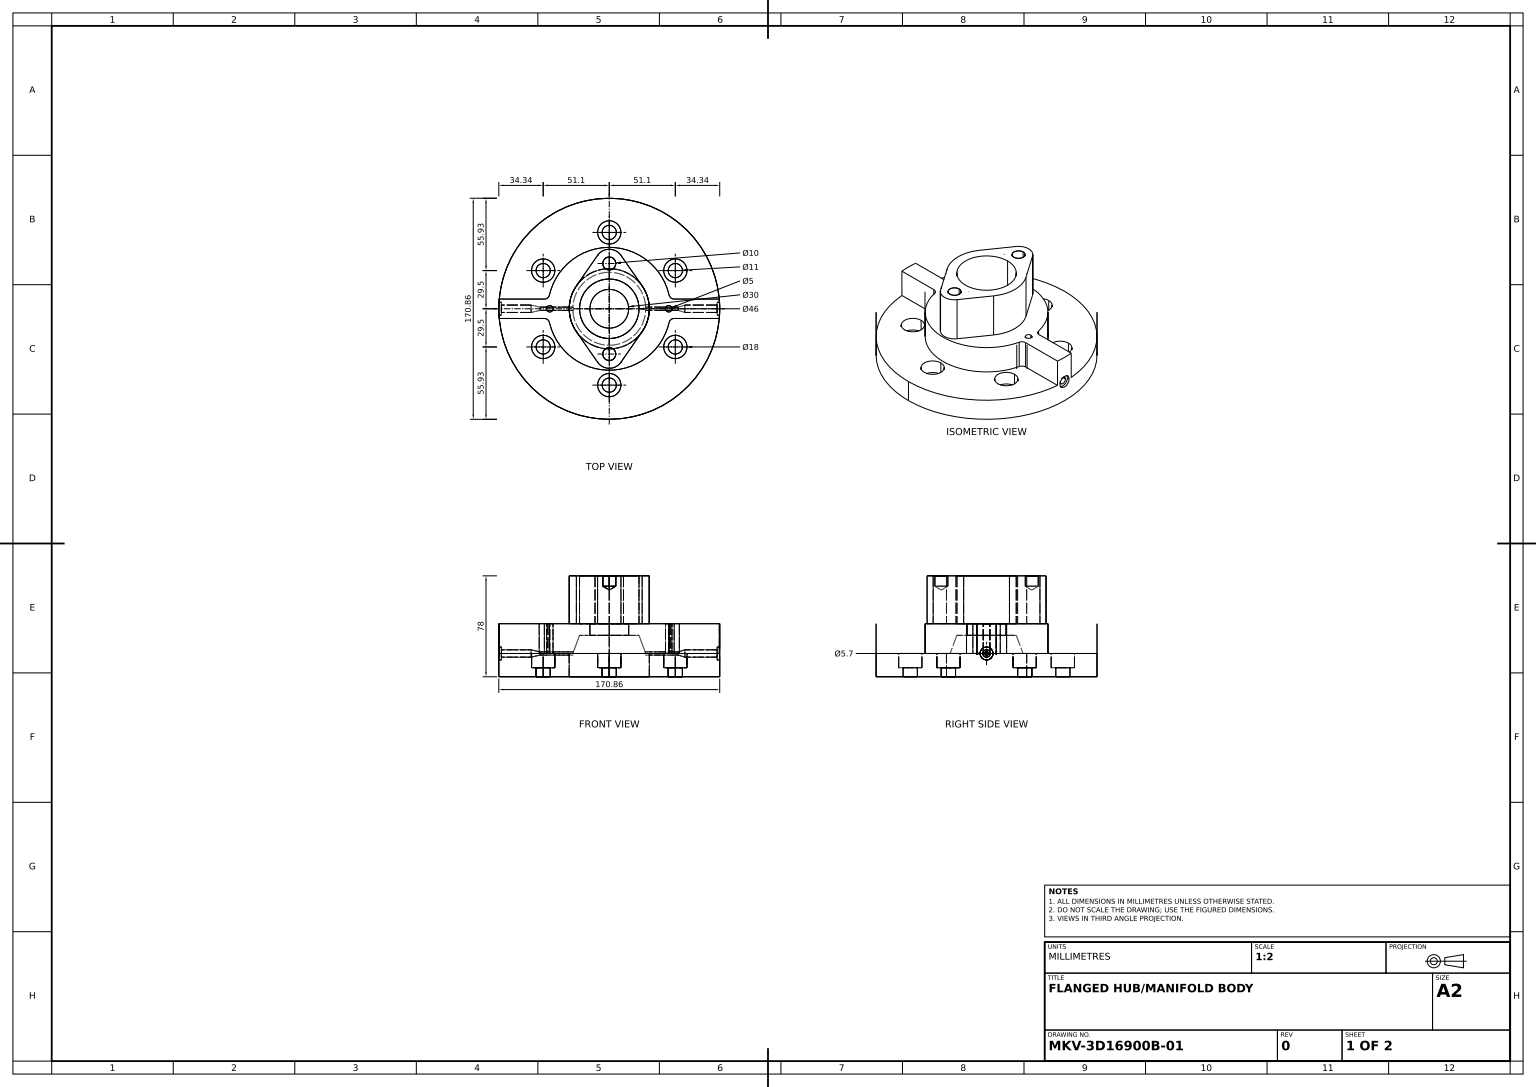
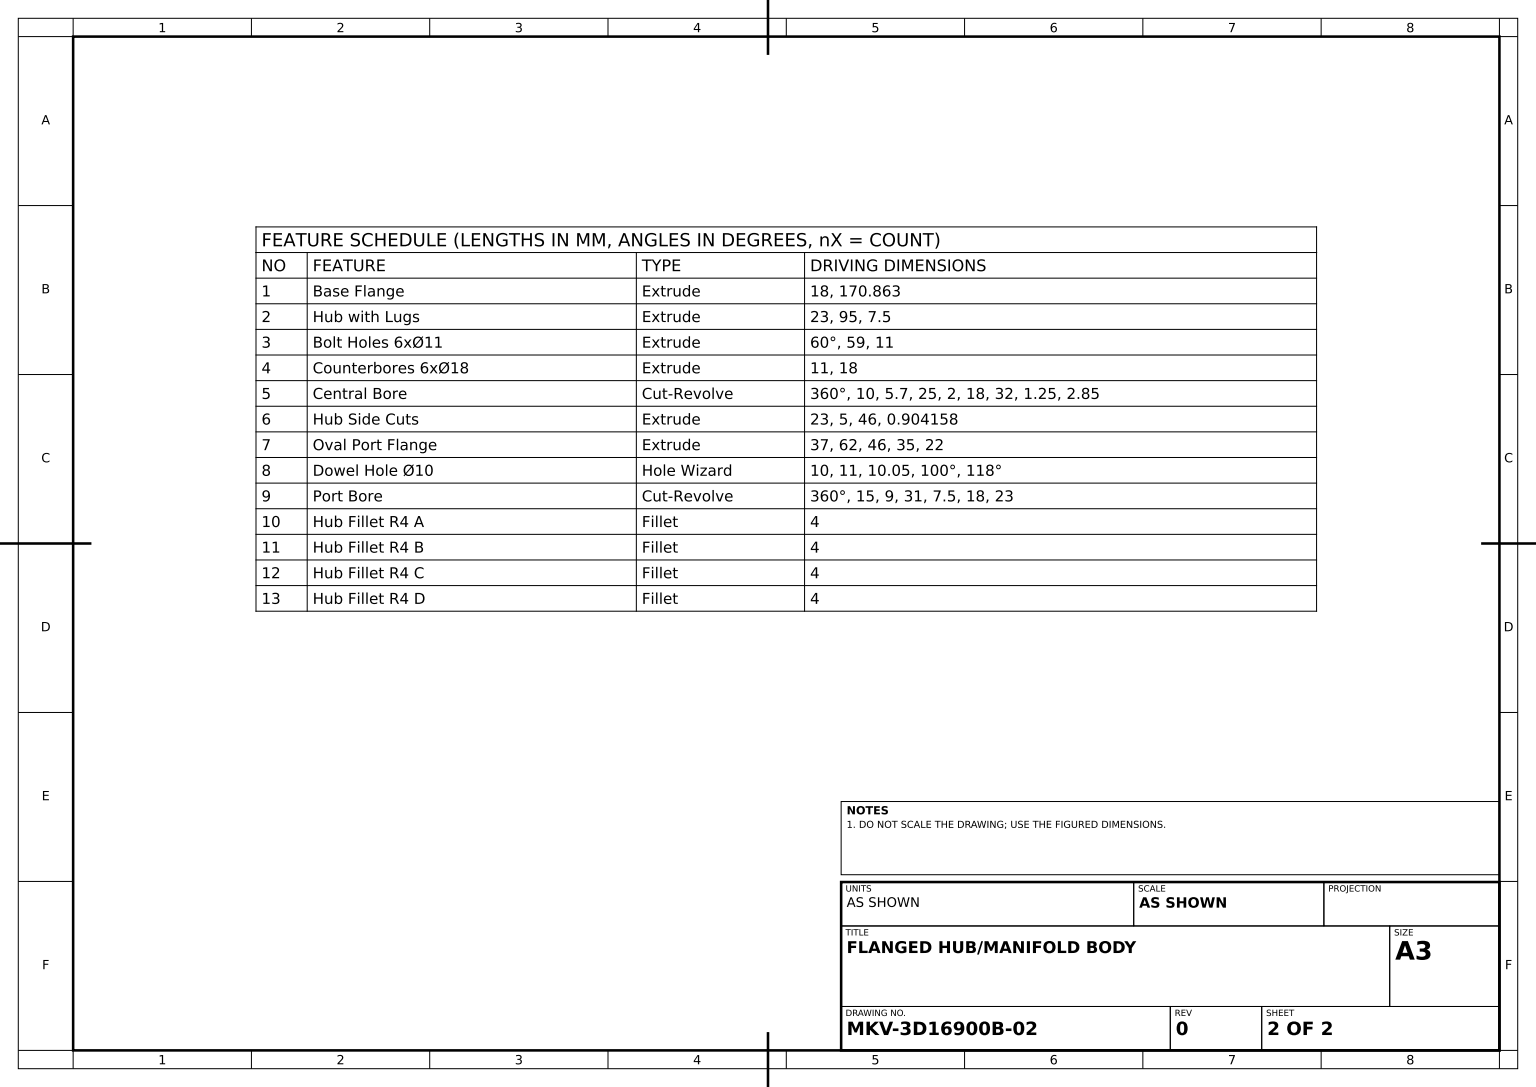
SolidWorks part; units mm, degrees
material "Plain Carbon Steel"
ref_plane "Front Plane" through (0, 0, 0) normal (0, 0, 1) x (1, 0, 0)
ref_plane "Top Plane" through (0, 0, 0) normal (0, 1, 0) x (1, 0, 0)
ref_plane "Right Plane" through (0, 0, 0) normal (1, 0, 0) x (0, 0, -1)
sketch "Base Flange Sketch" plane through (0, 0, 0) normal (0, 1, 0) x (1, 0, 0)
  circle A0 centre (0, 0) radius 85.4314
  dimension "D1" = 170.8628
extrude "Base Flange" add sketch "Base Flange Sketch" along normal blind 18
sketch "Hub with Lugs Sketch" plane through (0, 18, 0) normal (0, 1, 0) x (1, 0, 0)
  line L0 (-85.4314, 0) -> (85.4314, 0) construction
  line L1 (0, 85.4314) -> (0, -85.4314) construction
  line L2 (-46.9042, 7.5) -> (-85.1016, 7.5)
  line L3 (-46.9042, -7.5) -> (-85.1016, -7.5)
  line L4 (46.9042, 7.5) -> (85.1016, 7.5)
  line L5 (46.9042, -7.5) -> (85.1016, -7.5)
  arc A0 (-46.9042, -7.5) -> (46.9042, -7.5) centre (0, 0) ccw
  circle A1 centre (0, 0) radius 85.4314 construction
  arc A2 (-85.1016, 7.5) -> (-85.1016, -7.5) centre (0, 0) ccw
  arc A3 (85.1016, -7.5) -> (85.1016, 7.5) centre (0, 0) ccw
  arc A4 (46.9042, 7.5) -> (-46.9042, 7.5) centre (0, 0) ccw
  dimension "D1" = 95
  dimension "D2" = 7.5
  dimension "D3" = 7.5
  dimension "D4" = 7.5
  dimension "D5" = 7.5
extrude "Hub with Lugs" add sketch "Hub with Lugs Sketch" along normal blind 23
sketch "Bolt Holes Sketch" plane through (0, 18, 0) normal (0, 1, 0) x (1, 0, 0)
  line L0 (0, 85.4314) -> (0, -85.4314) construction
  line L1 (-85.4314, 0) -> (85.4314, 0) construction
  line L2 (0, 0) -> (-73.9858, 42.7157) construction
  line L3 (0, 0) -> (73.9858, -42.7157) construction
  line L4 (73.9858, 42.7157) -> (0, 0) construction
  line L5 (0, 0) -> (-75.3852, -43.5237) construction
  arc A0 (85.1016, 7.5) -> (-85.1016, 7.5) centre (0, 0) ccw construction
  arc A1 (-85.1016, -7.5) -> (85.1016, -7.5) centre (0, 0) ccw construction
  arc A2 (-85.1016, 7.5) -> (-85.1016, -7.5) centre (0, 0) ccw construction
  arc A3 (85.1016, -7.5) -> (85.1016, 7.5) centre (0, 0) ccw construction
  circle A6 centre (0, 59) radius 5.5
  circle A8 centre (0, -59) radius 5.5
  circle A10 centre (51.0955, 29.5) radius 5.5
  circle A12 centre (51.0955, -29.5) radius 5.5
  circle A14 centre (-51.0955, -29.5) radius 5.5
  circle A16 centre (-51.0955, 29.5) radius 5.5
  dimension "D12" = 11
  dimension "D13" = 11
  dimension "D14" = 11
  dimension "D15" = 11
  dimension "D16" = 11
  dimension "D17" = 11
  dimension "D1" = 60
  dimension "D2" = 60
  dimension "D3" = 60
  dimension "D4" = 60
  dimension "D5" = 59
  dimension "D6" = 59
  dimension "D7" = 59
  dimension "D8" = 59
  dimension "D9" = 59
  dimension "D10" = 59
extrude "Bolt Holes 6xØ11" cut sketch "Bolt Holes Sketch" against normal up to next
sketch "Counterbores Sketch" plane through (0, 18, 0) normal (0, 1, 0) x (1, 0, 0)
  circle A0 centre (0, 59) radius 9
  circle A1 centre (51.0955, 29.5) radius 9
  circle A2 centre (51.0955, -29.5) radius 9
  circle A3 centre (0, -59) radius 9
  circle A4 centre (-51.0955, -29.5) radius 9
  circle A5 centre (-51.0955, 29.5) radius 9
  dimension "D1" = 18
  dimension "D2" = 18
  dimension "D3" = 18
  dimension "D4" = 18
  dimension "D5" = 18
  dimension "D6" = 18
extrude "Counterbores 6xØ18" cut sketch "Counterbores Sketch" against normal blind 11
sketch "Central Bore Profile" plane through (0, 0, 0) normal (0, 0, 1) x (1, 0, 0)
  line L0 (-85.4314, 18) -> (-85.4314, 23)
  line L1 (-85.4314, 23) -> (-83.4314, 23)
  line L2 (-83.4314, 23) -> (-83.4314, 20.85)
  line L3 (-83.4314, 20.85) -> (-60.4314, 20.85)
  line L4 (-60.4314, 20.85) -> (-53.4314, 19.25)
  line L5 (-85.4314, 18) -> (-52.8119, 18) construction
  line L7 (85.4314, 18) -> (85.4314, 23)
  line L8 (85.4314, 0) -> (85.4314, 41) construction
  line L9 (85.4314, 23) -> (83.4314, 23)
  line L10 (83.4314, 23) -> (83.4314, 20.85)
  line L11 (83.4314, 20.85) -> (58.4314, 20.85)
  line L12 (58.4314, 20.85) -> (53.4314, 19.25)
  line L13 (85.4314, 18) -> (64.3325, 18) construction
  line L14 (85.1016, 18) -> (-85.1016, 18) construction
  line L15 (-53.4314, 19.25) -> (53.4314, 19.25)
  line L16 (-85.4314, 18) -> (85.4314, 18) construction
  line L17 (-85.4314, 18) -> (85.4314, 18)
  dimension "D1" = 10
  dimension "D2" = 5.7
  dimension "D3" = 25
  dimension "D4" = 2
  dimension "D5" = 32
  dimension "D6" = 1.25
  dimension "D7" = 18
  dimension "D8" = 10
  dimension "D9" = 32
  dimension "D10" = 2
  dimension "D11" = 1.25
  dimension "D12" = 2.85
  dimension "D13" = 25
revolve "Central Bore" cut sketch "Central Bore Profile" angle 360 about L17
sketch "Hub Side Cuts Sketch" plane through (0, 41, 0) normal (0, 1, 0) x (1, 0, 0)
  circle A0 centre (46, 0) radius 2.5
  circle A1 centre (-46, 0) radius 2.5
  dimension "D1" = 5
  dimension "D2" = 5
  dimension "D3" = 46
  dimension "D4" = 46
  dimension "D5" = 0.9042
extrude "Hub Side Cuts" cut sketch "Hub Side Cuts Sketch" against normal blind 23
sketch "Oval Port Flange Sketch" plane through (0, 41, 0) normal (0, 1, 0) x (1, 0, 0)
  line L0 (-9.0272, 41.2857) -> (-25.4402, 17.7143)
  line L1 (9.0272, 41.2857) -> (25.4402, 17.7143)
  line L2 (-9.0272, -41.2857) -> (-25.4402, -17.7143)
  line L3 (9.0272, -41.2857) -> (25.4402, -17.7143)
  arc A0 (25.4402, -17.7143) -> (25.4402, 17.7143) centre (0, 0) ccw
  circle A1 centre (0, 0) radius 23
  arc A2 (9.0272, 41.2857) -> (-9.0272, 41.2857) centre (0, 35) ccw
  arc A3 (-9.0272, -41.2857) -> (9.0272, -41.2857) centre (0, -35) ccw
  arc A4 (-25.4402, 17.7143) -> (-25.4402, -17.7143) centre (0, 0) ccw
  dimension "D1" = 62
  dimension "D2" = 46
  dimension "D5" = 22
  dimension "D6" = 22
  dimension "D3" = 35
  dimension "D4" = 35
extrude "Oval Port Flange" add sketch "Oval Port Flange Sketch" along normal blind 37
hole_wizard "Dowel Hole Ø10" positions "Sketch25" profile "Sketch26" hole size "Ø10.0" standard "ANSI Metric"
sketch "Sketch25" plane through (0, 78, 0) normal (0, 1, 0) x (1, 0, 0)
  point P0 (0, 35)
  point P3 (0, -35)
sketch "Sketch26" plane through (0, 78, -35) normal (1, 0, 0) x (0, 0, 1)
  line L0 (0, 0) -> (0, 11)
  line L1 (0, 11) -> (5, 7.9957)
  line L2 (5, 7.9957) -> (5, 0.021)
  line L3 (5, 0.021) -> (5.025, 0)
  line L5 (5.025, 0) -> (0, 0)
  line L6 (-5, 0.021) -> (-5.025, 0) construction
  line L10 (0, 11) -> (-5, 7.9957) construction
  line L11 (0, -6.35) -> (0, 107.95) construction
  dimension "Hole Dia." = 10
  dimension "Hole Depth" = 11
  dimension "Near C'Sink Dia." = 10.05
  dimension "Near C'Sink Angle" = 100
  dimension "Drill Angle" = 118
sketch "Port Bore Profile" plane through (0, 0, 0) normal (0, 0, 1) x (1, 0, 0)
  line L0 (0, 78) -> (0, 0) construction
  line L1 (9.0272, 78) -> (-9.0272, 78) construction
  line L2 (-28.1966, 18) -> (-31, 18)
  line L3 (0, 41) -> (-15, 41)
  line L4 (46.9042, 41) -> (-46.9042, 41) construction
  line L5 (-15, 41) -> (-15, 32)
  line L6 (-15, 32) -> (-23, 32)
  line L7 (0, 0) -> (0, 41)
  line L8 (85.1016, 18) -> (-85.1016, 18) construction
  line L9 (-31, 18) -> (-31, 0)
  line L10 (-85.4314, 0) -> (85.4314, 0) construction
  line L11 (-31, 0) -> (0, 0)
  line L12 (-28.1966, 18) -> (-23, 32)
  dimension "D1" = 15
  dimension "D2" = 9
  dimension "D3" = 31
  dimension "D4" = 7.5
  dimension "D5" = 23
  dimension "D6" = 18
revolve "Port Bore" cut sketch "Port Bore Profile" angle 360 about L0
fillet "Hub Fillet R4 A" radius 4 1 edges at (46.9042, 29.5, 7.5)
fillet "Hub Fillet R4 B" radius 4 1 edges at (46.9042, 29.5, -7.5)
fillet "Hub Fillet R4 C" radius 4 1 edges at (-46.9042, 29.5, -7.5)
fillet "Hub Fillet R4 D" radius 4 1 edges at (-46.9042, 29.5, 7.5)
